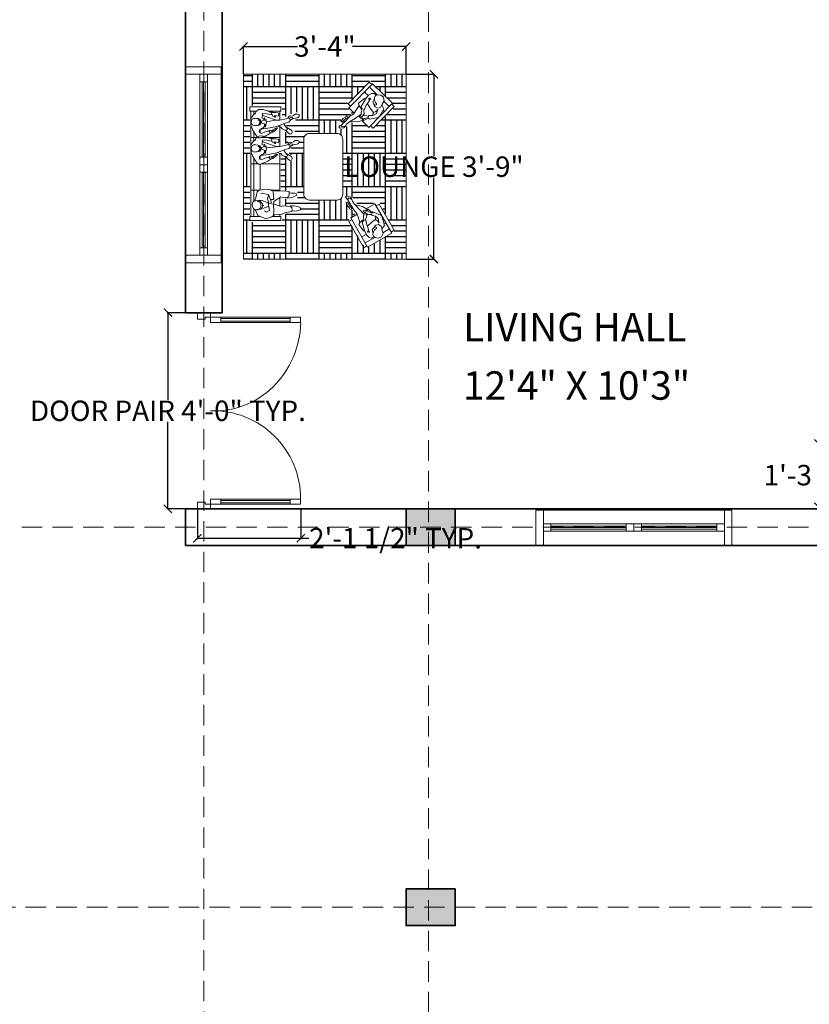
# Model space of a CAD drawing. Units: inches. Extents: x 782 to 2660, y -1008 to 166.
# Tile 3 of 12: x 1058 to 1251, y -598 to -357. Entities that reach past the tile are written whole.
import ezdxf

# ---------------------------------------------------------------- set-up
doc = ezdxf.new("R2010")
doc.units = ezdxf.units.IN
doc.header["$MEASUREMENT"] = 0
doc.linetypes.add('DASHED', pattern=[0.75, 0.5, -0.25])
for name, color, linetype, lineweight in [('A-ANNO-DIMS', 4, 'Continuous', 18), ('A-AREA-IDEN', 4, 'Continuous', 18), ('A-COLS', 7, 'Continuous', 35), ('A-Door', 150, 'Continuous', 18), ('A-FURN', 8, 'Continuous', 13), ('A-Glaz', 4, 'Continuous', 18), ('A-GRID', 8, 'DASHED', 13), ('A-WALL', 7, 'Continuous', 35)]:
    doc.layers.add(name, color=color, linetype=linetype, lineweight=lineweight)
doc.layers.add('NOITHAT', color=21, linetype='Continuous')
doc.styles.get("Standard").update_dxf_attribs({"font": 'arial.ttf'})
doc.dimstyles.get("Standard").update_dxf_attribs({"dimtxt": 5, "dimasz": 2, "dimexe": 0.18, "dimexo": 0.0625, "dimgap": 0.09, "dimtad": 0, "dimtih": 1, "dimtoh": 1, "dimdec": 0, "dimzin": 0, "dimdsep": 46, "dimlunit": 3, "dimtxsty": 'Standard', "dimblk": 'ARCHTICK', "dimcen": 0.09, "dimadec": 0, "dimazin": 0, "dimtfac": 1, "dimtdec": 0, "dimtofl": 0, "dimtmove": 0, "dimatfit": 3, "dimfxl": 1, "dimtolj": 1, "dimtzin": 0, "dimarcsym": 0})

# ---------------------------------------------------------------- blocks, each defined once
blk = doc.blocks.new('A$C13CE0A17')
at = {"layer": 'A-Door'}
for p, q in [((0, 0.61), (0, 0.69)), ((0, 0.69), (0.04, 0.69)), ((0.04, 0.69), (0.04, 0.61)), ((0, 0.61), (0, 0.08)), ((0.04, 0.61), (0, 0.61)), ((0.04, 0.61), (0, 0.61)), ((0.03, 0.61), (0.01, 0.61)), ((0.04, 0.08), (0.04, 0.61)), ((0, 0.08), (0, 0)), ((0.04, 0.08), (0, 0.08)), ((0, 0.08), (0.04, 0.08)), ((0.01, 0.08), (0.03, 0.08)), ((0.04, 0), (0.04, 0.08)), ((-0.035, 0), (-0.035, -0.1)), ((0, 0), (-0.035, 0)), ((0, 0), (0.04, 0)), ((0, -0.04), (0, 0)), ((0.015, -0.04), (0, -0.04)), ((0.015, -0.05), (0.015, -0.04)), ((0.015, -0.1), (0.015, -0.05)), ((-0.035, -0.1), (0.015, -0.1))]:
    blk.add_line(p, q, dxfattribs=at)
for points in [[(1.39, 0.69), (1.39, 0.61), (1.43, 0.61), (1.43, 0.69)], [(1.39, 0.08), (1.39, 0.61), (1.43, 0.61), (1.43, 0.08)], [(1.39, 0), (1.39, 0.08), (1.43, 0.08), (1.43, 0)], [(1.43, 0), (1.465, 0), (1.465, -0.1), (1.415, -0.1), (1.415, -0.05), (1.415, -0.04), (1.43, -0.04)]]:
    blk.add_lwpolyline(points, close=True, dxfattribs=at)
blk.add_arc((1.3872, 0.017), 0.673, 89.76573, 181.44381, dxfattribs=at)
blk.add_ellipse((0.0389, 0.0511), major_axis=(0.6669, -0.1217), ratio=0.940794, start_param=0.11153, end_param=1.73917, dxfattribs=at)
at = {"layer": 'A-Glaz'}
for p, q in [((0.01, 0.61), (0.01, 0.08)), ((0.03, 0.08), (0.03, 0.61))]:
    blk.add_line(p, q, dxfattribs=at)
blk.add_lwpolyline([(1.4, 0.08), (1.4, 0.61), (1.42, 0.61), (1.42, 0.08)], close=True, dxfattribs=at)
blk = doc.blocks.new('*X7')
at = {"color": 0}
for p, q in [((20100, 15000), (20100, 15102)), ((20200, 15000), (20200, 15102)), ((20300, 15000), (20300, 15102)), ((20400, 15000), (20400, 15102)), ((20400, 15100), (21000, 15100)), ((21000, 15000), (21000, 15102)), ((21100, 15000), (21100, 15102)), ((21200, 15000), (21200, 15102)), ((21300, 15000), (21300, 15102)), ((21400, 15000), (21400, 15102)), ((21500, 15000), (21500, 15102)), ((21600, 15000), (21600, 15102)), ((21600, 15100), (22200, 15100)), ((22200, 15000), (22200, 15102)), ((22300, 15000), (22300, 15102)), ((22400, 15000), (22400, 15102)), ((22500, 15000), (22500, 15102)), ((22600, 15000), (22600, 15102)), ((22700, 15000), (22700, 15102)), ((22800, 15000), (22800, 15102)), ((22800, 15100), (22953, 15100)), ((20023, 15000), (20400, 15000)), ((20400, 14703), (20400, 15000)), ((20400, 15000), (21000, 15000)), ((20500, 14764), (20500, 15000)), ((20600, 14825), (20600, 15000)), ((20700, 14886), (20700, 15000)), ((20800, 14850), (20800, 15000)), ((20900, 14679), (20900, 15000)), ((21000, 14509), (21000, 15000)), ((21000, 15000), (21600, 15000)), ((21600, 14400), (21600, 15000)), ((21600, 15000), (22200, 15000)), ((21700, 14400), (21700, 15000)), ((21800, 14400), (21800, 15000)), ((21900, 14400), (21900, 15000)), ((22000, 14400), (22000, 15000)), ((22100, 14400), (22100, 15000)), ((22200, 14400), (22200, 15000)), ((22200, 15000), (22800, 15000)), ((22800, 14436), (22800, 15000)), ((22800, 15000), (22953, 15000)), ((22900, 14400), (22900, 15000)), ((20023, 14900), (20400, 14900)), ((20023, 14800), (20400, 14800)), ((21000, 14900), (21600, 14900)), ((21000, 14800), (21600, 14800)), ((22200, 14900), (22800, 14900)), ((22200, 14800), (22800, 14800)), ((20023, 14700), (20395, 14700)), ((20023, 14600), (20239, 14600)), ((21000, 14700), (21600, 14700)), ((21000, 14600), (21600, 14600)), ((22200, 14700), (22800, 14700)), ((22200, 14600), (22800, 14600)), ((20023, 14500), (20290, 14500)), ((20023, 14400), (20341, 14400)), ((20100, 13800), (20100, 14400)), ((20200, 13800), (20200, 14400)), ((20300, 13800), (20300, 14400)), ((21005, 14500), (21600, 14500)), ((21048, 14400), (21600, 14400)), ((21100, 14103), (21100, 14400)), ((21200, 14013), (21200, 14400)), ((21300, 14038), (21300, 14400)), ((21400, 14038), (21400, 14400)), ((21500, 14038), (21500, 14400)), ((21600, 14038), (21600, 14400)), ((21600, 14400), (22200, 14400)), ((22200, 14500), (22800, 14500)), ((22200, 14301), (22200, 14400)), ((22200, 14400), (22258, 14400)), ((22840, 14400), (22953, 14400)), ((20400, 13800), (20400, 14284)), ((20400, 14200), (20443, 14200)), ((20948, 14300), (21000, 14300)), ((21000, 14220), (21000, 14352)), ((21600, 14300), (22196, 14300)), ((21600, 14200), (21914, 14200)), ((22840, 14300), (22953, 14300)), ((22840, 14200), (22953, 14200)), ((20400, 14100), (20493, 14100)), ((20615, 14100), (20911, 14100)), ((21600, 14100), (22200, 14100)), ((22200, 14013), (22200, 14136)), ((22840, 14100), (22953, 14100)), ((20400, 14000), (20986, 14000)), ((20400, 13900), (21000, 13900)), ((21000, 13800), (21000, 13985)), ((21100, 13800), (21100, 13955)), ((21846, 14000), (21984, 14000)), ((21867, 13900), (21984, 13900)), ((22200, 13800), (22200, 13872)), ((22840, 14000), (22953, 14000)), ((22840, 13900), (22953, 13900)), ((20023, 13800), (20400, 13800)), ((20023, 13700), (20400, 13700)), ((20400, 13200), (20400, 13800)), ((20400, 13800), (21000, 13800)), ((20500, 13200), (20500, 13800)), ((20600, 13200), (20600, 13800)), ((20700, 13200), (20700, 13800)), ((20800, 13200), (20800, 13800)), ((20900, 13200), (20900, 13800)), ((21000, 13200), (21000, 13800)), ((21000, 13800), (21167, 13800)), ((21000, 13700), (21167, 13700)), ((21867, 13800), (22200, 13800)), ((21900, 13200), (21900, 13800)), ((22000, 13200), (22000, 13800)), ((22100, 13337), (22100, 13800)), ((22200, 13278), (22200, 13800)), ((22200, 13800), (22284, 13800)), ((22200, 13700), (22284, 13700)), ((22840, 13800), (22953, 13800)), ((22900, 13200), (22900, 13800)), ((20023, 13600), (20400, 13600)), ((20023, 13500), (20400, 13500)), ((21000, 13600), (21167, 13600)), ((21000, 13500), (21167, 13500)), ((22200, 13600), (22284, 13600)), ((22200, 13500), (22284, 13500)), ((20023, 13400), (20400, 13400)), ((21000, 13400), (21167, 13400)), ((22200, 13400), (22284, 13400)), ((20023, 13300), (20400, 13300)), ((20023, 13200), (20400, 13200)), ((20100, 12600), (20100, 13200)), ((20200, 12600), (20200, 13200)), ((20300, 12600), (20300, 13200)), ((20400, 12600), (20400, 13200)), ((20400, 13200), (21000, 13200)), ((21000, 13300), (21167, 13300)), ((21000, 12645), (21000, 13200)), ((21000, 13200), (21167, 13200)), ((21100, 12710), (21100, 13200)), ((21867, 13200), (22129, 13200)), ((22100, 13200), (22100, 13222)), ((22200, 13300), (22284, 13300)), ((22840, 13200), (22953, 13200)), ((20400, 13100), (21000, 13100)), ((20400, 13000), (21000, 13000)), ((21867, 13100), (22104, 13100)), ((21867, 13000), (21940, 13000)), ((22158, 13000), (22200, 13000)), ((22200, 12812), (22200, 13017)), ((22840, 13100), (22953, 13100)), ((22840, 13000), (22953, 13000)), ((20400, 12900), (21000, 12900)), ((20400, 12800), (21000, 12800)), ((21200, 12760), (21200, 12864)), ((21300, 12600), (21300, 12838)), ((21400, 12600), (21400, 12838)), ((21500, 12600), (21500, 12838)), ((21600, 12600), (21600, 12838)), ((21600, 12800), (22032, 12800)), ((21859, 12900), (22200, 12900)), ((22840, 12900), (22953, 12900)), ((22840, 12800), (22953, 12800)), ((20023, 12600), (20400, 12600)), ((20400, 12700), (20570, 12700)), ((20400, 12536), (20400, 12600)), ((20400, 12600), (20466, 12600)), ((20745, 12700), (21000, 12700)), ((21194, 12600), (21600, 12600)), ((21200, 12600), (21200, 12607)), ((21600, 12700), (22177, 12700)), ((21600, 12000), (21600, 12600)), ((21600, 12600), (22019, 12600)), ((21700, 12000), (21700, 12600)), ((21800, 12000), (21800, 12600)), ((21900, 12000), (21900, 12600)), ((22000, 12592), (22000, 12600)), ((22840, 12700), (22953, 12700)), ((22840, 12600), (22953, 12600)), ((22900, 12000), (22900, 12600)), ((20023, 12500), (20362, 12500)), ((21000, 12457), (21000, 12480)), ((21025, 12500), (21600, 12500)), ((22000, 12000), (22000, 12457)), ((22100, 12000), (22100, 12483)), ((22200, 12000), (22200, 12534)), ((22200, 12500), (22258, 12500)), ((20023, 12400), (20258, 12400)), ((20023, 12300), (20265, 12300)), ((21057, 12400), (21600, 12400)), ((21082, 12300), (21600, 12300)), ((22200, 12400), (22258, 12400)), ((22200, 12300), (22800, 12300)), ((22800, 12000), (22800, 12337)), ((20023, 12200), (20363, 12200)), ((20023, 12100), (20400, 12100)), ((20400, 12000), (20400, 12163)), ((20900, 12000), (20900, 12118)), ((21000, 12000), (21000, 12218)), ((21000, 12200), (21600, 12200)), ((21000, 12100), (21600, 12100)), ((22200, 12200), (22800, 12200)), ((22200, 12100), (22800, 12100)), ((20023, 12000), (20400, 12000)), ((20100, 11772), (20100, 12000)), ((20200, 11772), (20200, 12000)), ((20300, 11772), (20300, 12000)), ((20400, 11772), (20400, 12000)), ((20400, 12000), (20560, 12000)), ((20400, 11900), (20658, 11900)), ((20500, 12000), (20500, 12061)), ((20682, 11900), (21000, 11900)), ((20782, 12000), (21000, 12000)), ((20800, 12000), (20800, 12018)), ((21000, 11772), (21000, 12000)), ((21000, 12000), (21600, 12000)), ((21100, 11772), (21100, 12000)), ((21200, 11772), (21200, 12000)), ((21300, 11772), (21300, 12000)), ((21400, 11772), (21400, 12000)), ((21500, 11772), (21500, 12000)), ((21600, 11772), (21600, 12000)), ((21600, 12000), (22200, 12000)), ((21600, 11900), (22200, 11900)), ((22200, 11772), (22200, 12000)), ((22200, 12000), (22800, 12000)), ((22300, 11772), (22300, 12000)), ((22400, 11772), (22400, 12000)), ((22500, 11772), (22500, 12000)), ((22600, 11772), (22600, 12000)), ((22700, 11772), (22700, 12000)), ((22800, 11772), (22800, 12000)), ((22800, 12000), (22953, 12000)), ((22800, 11900), (22953, 11900)), ((20400, 11800), (21000, 11800)), ((21600, 11800), (22200, 11800)), ((22800, 11800), (22953, 11800))]:
    blk.add_line(p, q, dxfattribs=at)
blk = doc.blocks.new('A$C47115F23')
at = {"linetype": 'ByBlock'}
for p, q in [((693, 2256), (693, 2818)), ((693, 2818), (768, 2818)), ((728, 2530), (788, 2676)), ((768, 2629), (768, 2818)), ((768, 2800), (2668, 2800)), ((768, 2743), (908, 2743)), ((788, 2676), (884, 2718)), ((890, 2723), (888, 2688)), ((888, 2688), (898, 2620)), ((890, 2723), (914, 2751)), ((892, 2687), (904, 2639)), ((914, 2751), (946, 2771)), ((946, 2771), (985, 2775)), ((985, 2775), (1037, 2759)), ((1027, 2639), (1039, 2683)), ((1039, 2683), (1035, 2648)), ((1056, 2700), (1037, 2759)), ((1042, 2743), (1815, 2743)), ((1049, 2650), (1056, 2700)), ((1072, 2723), (1050, 2729)), ((1056, 2593), (1061, 2665)), ((1072, 2723), (1104, 2707)), ((1104, 2707), (1210, 2684)), ((1210, 2684), (1242, 2652)), ((1243, 2800), (1243, 2644)), ((1710, 2662), (1709, 2626)), ((1729, 2684), (1710, 2662)), ((1718, 2800), (1718, 2671)), ((1790, 2728), (1729, 2684)), ((1846, 2763), (1790, 2728)), ((1893, 2783), (1846, 2763)), ((1939, 2797), (1893, 2783)), ((1928, 2739), (1930, 2714)), ((1932, 2739), (1928, 2739)), ((1930, 2714), (1932, 2685)), ((1933, 2750), (1932, 2739)), ((1932, 2685), (1939, 2656)), ((1942, 2777), (1933, 2750)), ((1979, 2802), (1939, 2797)), ((1952, 2655), (1940, 2668)), ((1964, 2790), (1942, 2777)), ((1994, 2795), (1964, 2790)), ((2047, 2799), (1979, 2802)), ((2021, 2790), (1994, 2795)), ((2045, 2777), (2021, 2790)), ((2030, 2672), (2026, 2650)), ((2036, 2650), (2030, 2672)), ((2042, 2640), (2056, 2669)), ((2055, 2756), (2045, 2777)), ((2082, 2783), (2047, 2799)), ((2059, 2741), (2055, 2756)), ((2056, 2669), (2059, 2712)), ((2064, 2736), (2059, 2741)), ((2059, 2712), (2064, 2736)), ((2118, 2755), (2082, 2783)), ((2152, 2716), (2118, 2755)), ((2127, 2743), (2290, 2743)), ((2179, 2707), (2152, 2716)), ((2196, 2692), (2179, 2707)), ((2185, 2662), (2184, 2626)), ((2204, 2684), (2185, 2662)), ((2193, 2800), (2193, 2694)), ((2193, 2800), (2193, 2671)), ((2218, 2658), (2196, 2692)), ((2265, 2728), (2204, 2684)), ((2321, 2763), (2265, 2728)), ((2368, 2783), (2321, 2763)), ((2414, 2797), (2368, 2783)), ((2403, 2739), (2405, 2714)), ((2407, 2739), (2403, 2739)), ((2405, 2714), (2407, 2685)), ((2408, 2750), (2407, 2739)), ((2407, 2685), (2414, 2656)), ((2417, 2777), (2408, 2750)), ((2454, 2802), (2414, 2797)), ((2427, 2655), (2415, 2668)), ((2439, 2790), (2417, 2777)), ((2469, 2795), (2439, 2790)), ((2522, 2799), (2454, 2802)), ((2496, 2790), (2469, 2795)), ((2520, 2777), (2496, 2790)), ((2505, 2672), (2501, 2650)), ((2511, 2650), (2505, 2672)), ((2517, 2640), (2531, 2669)), ((2530, 2756), (2520, 2777)), ((2557, 2783), (2522, 2799)), ((2534, 2741), (2530, 2756)), ((2531, 2669), (2534, 2712)), ((2539, 2736), (2534, 2741)), ((2534, 2712), (2539, 2736)), ((2593, 2755), (2557, 2783)), ((2627, 2716), (2593, 2755)), ((2602, 2743), (2668, 2743)), ((2654, 2707), (2627, 2716)), ((2671, 2692), (2654, 2707)), ((2668, 2818), (2668, 2694)), ((2668, 2818), (2743, 2818)), ((2693, 2658), (2671, 2692)), ((2743, 2818), (2743, 2256)), ((760, 2423), (728, 2530)), ((768, 2631), (769, 2631)), ((867, 2553), (843, 2518)), ((843, 2518), (874, 2463)), ((874, 2463), (1011, 2485)), ((896, 2631), (921, 2631)), ((898, 2620), (927, 2598)), ((904, 2639), (960, 2612)), ((911, 2583), (946, 2485)), ((927, 2598), (955, 2589)), ((955, 2589), (963, 2573)), ((960, 2612), (1003, 2624)), ((963, 2573), (968, 2573)), ((968, 2573), (977, 2590)), ((977, 2590), (1002, 2598)), ((1011, 2485), (989, 2391)), ((1002, 2598), (1031, 2619)), ((1003, 2624), (1027, 2639)), ((1011, 2476), (1056, 2593)), ((1088, 2498), (1011, 2476)), ((1014, 2631), (1059, 2631)), ((1031, 2619), (1049, 2650)), ((1035, 2648), (1043, 2643)), ((1155, 2482), (1088, 2498)), ((1163, 2482), (1187, 2621)), ((1242, 2652), (1262, 2530)), ((1246, 2631), (1718, 2631)), ((1262, 2530), (1250, 2447)), ((1709, 2626), (1742, 2555)), ((1718, 2605), (1718, 2275)), ((1742, 2555), (1764, 2496)), ((1764, 2496), (1783, 2467)), ((1786, 2616), (1802, 2640)), ((1803, 2584), (1786, 2616)), ((1796, 2631), (1860, 2631)), ((1802, 2640), (1825, 2648)), ((1827, 2524), (1803, 2584)), ((1825, 2648), (1849, 2646)), ((1832, 2494), (1827, 2524)), ((1829, 2482), (1832, 2494)), ((1849, 2646), (1874, 2612)), ((1883, 2606), (1869, 2602)), ((1869, 2602), (1871, 2575)), ((1871, 2575), (1879, 2526)), ((1874, 2612), (1883, 2606)), ((1879, 2592), (1881, 2599)), ((1896, 2574), (1879, 2592)), ((1879, 2526), (1915, 2333)), ((1923, 2553), (1896, 2574)), ((1933, 2530), (1903, 2545)), ((1957, 2553), (1923, 2553)), ((1952, 2536), (1933, 2530)), ((1939, 2656), (1947, 2638)), ((1947, 2638), (1962, 2626)), ((1972, 2642), (1952, 2655)), ((1956, 2631), (2028, 2631)), ((1957, 2540), (1979, 2614)), ((1959, 2523), (1957, 2540)), ((1972, 2629), (1959, 2635)), ((2003, 2516), (1959, 2523)), ((1962, 2626), (1981, 2622)), ((1996, 2638), (1972, 2642)), ((1981, 2622), (1990, 2608)), ((1990, 2608), (1998, 2609)), ((2013, 2641), (1996, 2638)), ((1998, 2609), (2005, 2624)), ((2035, 2538), (2003, 2516)), ((2005, 2624), (2023, 2628)), ((2010, 2455), (2005, 2513)), ((2029, 2635), (2008, 2630)), ((2026, 2650), (2013, 2641)), ((2013, 2623), (2016, 2590)), ((2016, 2590), (2025, 2560)), ((2018, 2528), (2040, 2521)), ((2023, 2628), (2042, 2640)), ((2025, 2560), (2033, 2555)), ((2057, 2580), (2033, 2567)), ((2033, 2555), (2035, 2538)), ((2050, 2660), (2036, 2650)), ((2040, 2541), (2055, 2546)), ((2043, 2379), (2113, 2584)), ((2055, 2546), (2069, 2558)), ((2072, 2599), (2057, 2580)), ((2087, 2596), (2072, 2599)), ((2111, 2589), (2087, 2596)), ((2113, 2584), (2128, 2594)), ((2141, 2519), (2125, 2428)), ((2128, 2594), (2148, 2585)), ((2148, 2585), (2141, 2519)), ((2184, 2626), (2217, 2555)), ((2190, 2482), (2218, 2577)), ((2193, 2605), (2193, 2275)), ((2193, 2492), (2193, 2275)), ((2217, 2555), (2239, 2496)), ((2223, 2616), (2218, 2658)), ((2218, 2577), (2223, 2616)), ((2239, 2496), (2258, 2467)), ((2261, 2616), (2277, 2640)), ((2278, 2584), (2261, 2616)), ((2271, 2631), (2335, 2631)), ((2277, 2640), (2300, 2648)), ((2302, 2524), (2278, 2584)), ((2300, 2648), (2324, 2646)), ((2307, 2494), (2302, 2524)), ((2304, 2482), (2307, 2494)), ((2324, 2646), (2349, 2612)), ((2358, 2606), (2344, 2602)), ((2344, 2602), (2346, 2575)), ((2346, 2575), (2354, 2526)), ((2349, 2612), (2358, 2606)), ((2354, 2592), (2356, 2599)), ((2371, 2574), (2354, 2592)), ((2354, 2526), (2390, 2333)), ((2398, 2553), (2371, 2574)), ((2408, 2530), (2378, 2545)), ((2432, 2553), (2398, 2553)), ((2427, 2536), (2408, 2530)), ((2414, 2656), (2422, 2638)), ((2422, 2638), (2437, 2626)), ((2447, 2642), (2427, 2655)), ((2431, 2631), (2503, 2631)), ((2432, 2540), (2454, 2614)), ((2434, 2523), (2432, 2540)), ((2447, 2629), (2434, 2635)), ((2478, 2516), (2434, 2523)), ((2437, 2626), (2456, 2622)), ((2471, 2638), (2447, 2642)), ((2456, 2622), (2465, 2608)), ((2465, 2608), (2473, 2609)), ((2488, 2641), (2471, 2638)), ((2473, 2609), (2480, 2624)), ((2510, 2538), (2478, 2516)), ((2480, 2624), (2498, 2628)), ((2485, 2455), (2480, 2513)), ((2504, 2635), (2483, 2630)), ((2501, 2650), (2488, 2641)), ((2488, 2623), (2491, 2590)), ((2491, 2590), (2500, 2560)), ((2493, 2528), (2515, 2521)), ((2498, 2628), (2517, 2640)), ((2500, 2560), (2508, 2555)), ((2532, 2580), (2508, 2567)), ((2508, 2555), (2510, 2538)), ((2525, 2660), (2511, 2650)), ((2515, 2541), (2530, 2546)), ((2518, 2379), (2588, 2584)), ((2530, 2546), (2544, 2558)), ((2547, 2599), (2532, 2580)), ((2562, 2596), (2547, 2599)), ((2586, 2589), (2562, 2596)), ((2588, 2584), (2603, 2594)), ((2616, 2519), (2600, 2428)), ((2603, 2594), (2623, 2585)), ((2623, 2585), (2616, 2519)), ((2665, 2482), (2693, 2577)), ((2668, 2492), (2668, 2256)), ((2698, 2616), (2693, 2658)), ((2693, 2577), (2698, 2616)), ((795, 2376), (760, 2423)), ((768, 2256), (768, 2412)), ((851, 2384), (795, 2391)), ((811, 2241), (795, 2376)), ((989, 2391), (851, 2384)), ((993, 2388), (950, 2245)), ((1040, 2388), (993, 2388)), ((1068, 2439), (1013, 2435)), ((1120, 2257), (1040, 2388)), ((1072, 2388), (1076, 2443)), ((1210, 2399), (1072, 2388)), ((1076, 2443), (1163, 2482)), ((1230, 2415), (1222, 2301)), ((1250, 2447), (1230, 2415)), ((1243, 2436), (1243, 2275)), ((1783, 2467), (1797, 2442)), ((1797, 2442), (1805, 2440)), ((1803, 2443), (1808, 2457)), ((1805, 2440), (1813, 2403)), ((1808, 2457), (1822, 2464)), ((1813, 2403), (1846, 2355)), ((1830, 2419), (1819, 2423)), ((1822, 2464), (1837, 2458)), ((1839, 2469), (1829, 2482)), ((1838, 2407), (1830, 2419)), ((1835, 2447), (1846, 2453)), ((1842, 2435), (1835, 2447)), ((1844, 2401), (1838, 2407)), ((1846, 2453), (1839, 2469)), ((1849, 2418), (1842, 2435)), ((1849, 2405), (1844, 2401)), ((1846, 2355), (1886, 2320)), ((1851, 2408), (1849, 2418)), ((1857, 2389), (1851, 2408)), ((1876, 2355), (1857, 2389)), ((1888, 2338), (1876, 2355)), ((1891, 2325), (1879, 2340)), ((1879, 2340), (1888, 2338)), ((1886, 2320), (1891, 2325)), ((1901, 2277), (1915, 2308)), ((1915, 2333), (1942, 2262)), ((2020, 2384), (2010, 2455)), ((2028, 2326), (2020, 2384)), ((2030, 2330), (2043, 2379)), ((2030, 2277), (2030, 2330)), ((2103, 2404), (2084, 2365)), ((2084, 2365), (2084, 2355)), ((2084, 2355), (2089, 2354)), ((2089, 2354), (2108, 2372)), ((2128, 2413), (2103, 2404)), ((2114, 2372), (2103, 2301)), ((2108, 2372), (2114, 2372)), ((2125, 2428), (2128, 2413)), ((2131, 2426), (2147, 2429)), ((2147, 2429), (2171, 2413)), ((2162, 2306), (2165, 2350)), ((2165, 2350), (2167, 2404)), ((2167, 2404), (2175, 2408)), ((2175, 2452), (2190, 2482)), ((2175, 2408), (2175, 2452)), ((2258, 2467), (2272, 2442)), ((2272, 2442), (2280, 2440)), ((2278, 2443), (2283, 2457)), ((2280, 2440), (2288, 2403)), ((2283, 2457), (2297, 2464)), ((2288, 2403), (2321, 2355)), ((2305, 2419), (2294, 2423)), ((2297, 2464), (2312, 2458)), ((2314, 2469), (2304, 2482)), ((2313, 2407), (2305, 2419)), ((2310, 2447), (2321, 2453)), ((2317, 2435), (2310, 2447)), ((2319, 2401), (2313, 2407)), ((2321, 2453), (2314, 2469)), ((2324, 2418), (2317, 2435)), ((2324, 2405), (2319, 2401)), ((2321, 2355), (2361, 2320)), ((2326, 2408), (2324, 2418)), ((2332, 2389), (2326, 2408)), ((2351, 2355), (2332, 2389)), ((2363, 2338), (2351, 2355)), ((2366, 2325), (2354, 2340)), ((2354, 2340), (2363, 2338)), ((2361, 2320), (2366, 2325)), ((2376, 2277), (2390, 2308)), ((2390, 2333), (2417, 2262)), ((2495, 2384), (2485, 2455)), ((2503, 2326), (2495, 2384)), ((2505, 2330), (2518, 2379)), ((2505, 2277), (2505, 2330)), ((2578, 2404), (2559, 2365)), ((2559, 2365), (2559, 2355)), ((2559, 2355), (2564, 2354)), ((2564, 2354), (2583, 2372)), ((2603, 2413), (2578, 2404)), ((2589, 2372), (2578, 2301)), ((2583, 2372), (2589, 2372)), ((2600, 2428), (2603, 2413)), ((2606, 2426), (2622, 2429)), ((2622, 2429), (2646, 2413)), ((2637, 2306), (2640, 2350)), ((2640, 2350), (2642, 2404)), ((2642, 2404), (2650, 2408)), ((2650, 2452), (2665, 2482)), ((2650, 2408), (2650, 2452)), ((768, 2256), (693, 2256)), ((807, 2275), (768, 2275)), ((835, 2186), (811, 2241)), ((859, 2068), (835, 2186)), ((950, 2245), (957, 2222)), ((957, 2222), (950, 2091)), ((1109, 2275), (959, 2275)), ((1096, 2135), (1116, 2151)), ((1116, 2044), (1096, 2135)), ((1112, 2230), (1120, 2257)), ((1116, 2151), (1112, 2230)), ((1124, 2123), (1112, 2170)), ((1230, 2210), (1218, 2111)), ((1222, 2301), (1230, 2210)), ((1902, 2275), (1225, 2275)), ((1798, 2125), (1830, 2156)), ((1830, 2156), (1844, 2172)), ((1896, 2150), (1844, 2062)), ((1846, 2186), (1871, 2232)), ((1846, 2157), (1846, 2186)), ((1856, 2147), (1846, 2157)), ((1874, 2140), (1856, 2147)), ((1871, 2232), (1903, 2260)), ((1901, 2161), (1874, 2140)), ((1903, 2260), (1901, 2277)), ((1959, 2206), (1901, 2161)), ((1942, 2262), (1967, 2198)), ((1967, 2198), (1993, 2112)), ((2054, 2164), (2030, 2277)), ((2412, 2275), (2030, 2275)), ((2065, 2125), (2054, 2164)), ((2103, 2301), (2113, 2301)), ((2113, 2301), (2118, 2284)), ((2118, 2284), (2123, 2288)), ((2123, 2288), (2131, 2296)), ((2131, 2296), (2141, 2298)), ((2141, 2298), (2147, 2303)), ((2147, 2303), (2162, 2306)), ((2273, 2125), (2305, 2156)), ((2305, 2156), (2319, 2172)), ((2371, 2150), (2319, 2062)), ((2321, 2186), (2346, 2232)), ((2321, 2157), (2321, 2186)), ((2331, 2147), (2321, 2157)), ((2349, 2140), (2331, 2147)), ((2346, 2232), (2378, 2260)), ((2376, 2161), (2349, 2140)), ((2378, 2260), (2376, 2277)), ((2434, 2206), (2376, 2161)), ((2417, 2262), (2442, 2198)), ((2442, 2198), (2468, 2112)), ((2529, 2164), (2505, 2277)), ((2668, 2275), (2505, 2275)), ((2540, 2125), (2529, 2164)), ((2578, 2301), (2588, 2301)), ((2588, 2301), (2593, 2284)), ((2593, 2284), (2598, 2288)), ((2598, 2288), (2606, 2296)), ((2606, 2296), (2616, 2298)), ((2616, 2298), (2622, 2303)), ((2622, 2303), (2637, 2306)), ((2668, 2256), (2743, 2256)), ((874, 2056), (859, 2068)), ((889, 1903), (861, 1982)), ((863, 1981), (867, 2044)), ((867, 2044), (874, 2056)), ((924, 2063), (894, 2054)), ((946, 1953), (922, 1902)), ((945, 2083), (924, 2063)), ((957, 2032), (946, 1953)), ((950, 2091), (957, 2079)), ((957, 2079), (957, 2032)), ((1151, 1969), (1116, 2044)), ((1159, 2107), (1124, 2123)), ((1179, 1977), (1151, 1969)), ((1191, 2107), (1159, 2107)), ((1187, 2008), (1179, 1977)), ((1195, 2107), (1187, 2068)), ((1187, 2068), (1187, 2008)), ((1218, 2111), (1195, 2107)), ((1778, 2096), (1798, 2125)), ((1783, 2069), (1778, 2096)), ((1808, 2052), (1783, 2069)), ((1844, 2062), (1808, 2052)), ((1993, 2112), (2030, 2086)), ((2030, 2086), (2055, 2049)), ((2042, 2090), (2057, 2105)), ((2055, 2049), (2059, 2025)), ((2057, 2105), (2062, 2120)), ((2057, 2040), (2074, 2056)), ((2059, 2025), (2076, 1946)), ((2082, 2125), (2065, 2125)), ((2079, 2091), (2070, 2103)), ((2074, 2056), (2081, 2076)), ((2081, 2076), (2079, 2091)), ((2099, 2106), (2082, 2125)), ((2109, 2076), (2099, 2106)), ((2103, 2069), (2109, 2076)), ((2113, 2032), (2103, 2069)), ((2135, 2000), (2113, 2032)), ((2128, 1929), (2138, 1954)), ((2138, 1954), (2135, 2000)), ((2253, 2096), (2273, 2125)), ((2258, 2069), (2253, 2096)), ((2283, 2052), (2258, 2069)), ((2319, 2062), (2283, 2052)), ((2468, 2112), (2505, 2086)), ((2505, 2086), (2530, 2049)), ((2517, 2090), (2532, 2105)), ((2530, 2049), (2534, 2025)), ((2532, 2105), (2537, 2120)), ((2532, 2040), (2549, 2056)), ((2534, 2025), (2551, 1946)), ((2557, 2125), (2540, 2125)), ((2554, 2091), (2545, 2103)), ((2549, 2056), (2556, 2076)), ((2556, 2076), (2554, 2091)), ((2574, 2106), (2557, 2125)), ((2584, 2076), (2574, 2106)), ((2578, 2069), (2584, 2076)), ((2588, 2032), (2578, 2069)), ((2610, 2000), (2588, 2032)), ((2603, 1929), (2613, 1954)), ((2613, 1954), (2610, 2000)), ((922, 1902), (890, 1902)), ((2076, 1946), (2101, 1927)), ((2101, 1927), (2128, 1929)), ((2551, 1946), (2576, 1927)), ((2576, 1927), (2603, 1929)), ((1023, 1080), (953, 1052)), ((1025, 1059), (1023, 1080)), ((1093, 1075), (1069, 1049)), ((1120, 1091), (1093, 1075)), ((1114, 1001), (1142, 1069)), ((1142, 1069), (1120, 1091)), ((2357, 1196), (2383, 1212)), ((2367, 1123), (2357, 1196)), ((2387, 1102), (2367, 1123)), ((2383, 1212), (2406, 1190)), ((2395, 1164), (2386, 1156)), ((2386, 1156), (2390, 1128)), ((2406, 1090), (2387, 1102)), ((2390, 1128), (2402, 1088)), ((2414, 1159), (2395, 1164)), ((2406, 1190), (2422, 1158)), ((2429, 1075), (2406, 1090)), ((2422, 1158), (2448, 1136)), ((2471, 1023), (2429, 1075)), ((2448, 1136), (2479, 1101)), ((2468, 1157), (2475, 1177)), ((2483, 1131), (2468, 1157)), ((2475, 1177), (2536, 1133)), ((2479, 1101), (2483, 1131)), ((2547, 1039), (2479, 1101)), ((2533, 1090), (2491, 1130)), ((2549, 1052), (2533, 1090)), ((2536, 1133), (2560, 1094)), ((2560, 1094), (2581, 1077)), ((2581, 1077), (2570, 1052)), ((678, 1034), (205, 761)), ((746, 1000), (218, 696)), ((710, 979), (678, 1034)), ((812, 885), (746, 1000)), ((824, 889), (759, 867)), ((886, 946), (824, 889)), ((919, 964), (886, 946)), ((892, 841), (988, 930)), ((919, 1020), (895, 1009)), ((895, 1009), (900, 983)), ((900, 983), (919, 964)), ((953, 1052), (919, 1020)), ((919, 964), (999, 1007)), ((920, 977), (945, 1010)), ((945, 1010), (995, 1039)), ((960, 842), (980, 912)), ((980, 912), (988, 930)), ((988, 930), (1042, 969)), ((999, 1007), (1003, 1037)), ((1039, 1034), (999, 1007)), ((1003, 1037), (1025, 1059)), ((1069, 1049), (1039, 1034)), ((1042, 969), (1068, 978)), ((1068, 978), (1089, 985)), ((1093, 1011), (1071, 976)), ((1078, 1047), (1097, 1047)), ((1089, 985), (1114, 1001)), ((1103, 1037), (1093, 1011)), ((1097, 1047), (1103, 1037)), ((2475, 1004), (2471, 1023)), ((2542, 914), (2472, 1023)), ((2477, 931), (2475, 1004)), ((2475, 877), (2477, 931)), ((2604, 816), (2542, 914)), ((2570, 1052), (2547, 1039)), ((2547, 1039), (2574, 1013)), ((2574, 1013), (2620, 942)), ((2620, 942), (2677, 905)), ((2630, 936), (2723, 1031)), ((2677, 905), (2770, 850)), ((2723, 1031), (3159, 606)), ((2753, 1002), (2797, 1047)), ((2797, 1047), (3188, 665)), ((205, 761), (237, 707)), ((291, 738), (389, 568)), ((436, 718), (392, 666)), ((446, 722), (400, 801)), ((503, 748), (436, 718)), ((510, 771), (503, 748)), ((623, 856), (510, 771)), ((664, 792), (518, 750)), ((534, 677), (621, 710)), ((621, 710), (708, 725)), ((655, 836), (623, 856)), ((759, 867), (655, 836)), ((664, 830), (709, 776)), ((697, 766), (664, 792)), ((770, 768), (697, 766)), ((704, 738), (809, 700)), ((708, 725), (704, 738)), ((848, 752), (770, 768)), ((790, 720), (850, 736)), ((819, 707), (790, 720)), ((808, 763), (892, 841)), ((838, 783), (855, 774)), ((850, 736), (848, 752)), ((855, 774), (874, 755)), ((869, 730), (861, 713)), ((861, 713), (887, 722)), ((893, 717), (862, 689)), ((874, 755), (869, 730)), ((887, 722), (893, 717)), ((893, 698), (948, 789)), ((998, 564), (907, 721)), ((948, 789), (960, 842)), ((2371, 671), (2498, 801)), ((2506, 775), (2475, 877)), ((2497, 767), (2506, 775)), ((2540, 675), (2497, 767)), ((2518, 796), (2511, 793)), ((2511, 793), (2534, 758)), ((2540, 781), (2518, 796)), ((2534, 758), (2549, 683)), ((2538, 826), (2537, 800)), ((2537, 800), (2540, 781)), ((2561, 839), (2538, 826)), ((2557, 801), (2563, 816)), ((2611, 770), (2557, 801)), ((2580, 843), (2561, 839)), ((2563, 816), (2642, 812)), ((2576, 677), (2585, 735)), ((2580, 765), (2611, 770)), ((2588, 756), (2580, 765)), ((2699, 766), (2588, 756)), ((2642, 812), (2712, 793)), ((2691, 755), (2699, 766)), ((2772, 719), (2691, 755)), ((2760, 846), (2703, 805)), ((2712, 793), (2751, 809)), ((2751, 809), (2882, 733)), ((2770, 850), (2807, 861)), ((2848, 665), (2772, 719)), ((2807, 861), (2895, 751)), ((2895, 751), (2896, 727)), ((2896, 727), (2953, 681)), ((2945, 687), (3009, 752)), ((218, 696), (470, 260)), ((389, 568), (377, 502)), ((392, 666), (379, 624)), ((379, 624), (399, 575)), ((399, 575), (389, 568)), ((423, 595), (404, 581)), ((452, 601), (423, 595)), ((486, 590), (452, 601)), ((469, 598), (532, 612)), ((470, 260), (998, 564)), ((475, 669), (511, 666)), ((511, 666), (485, 700)), ((485, 700), (534, 677)), ((529, 571), (486, 590)), ((550, 536), (529, 571)), ((532, 612), (566, 581)), ((567, 533), (550, 536)), ((566, 581), (579, 562)), ((586, 571), (567, 533)), ((611, 547), (586, 571)), ((591, 695), (672, 615)), ((623, 500), (611, 547)), ((672, 615), (715, 553)), ((715, 553), (688, 517)), ((715, 553), (769, 555)), ((720, 497), (772, 552)), ((772, 552), (792, 623)), ((779, 437), (850, 598)), ((792, 623), (818, 613)), ((801, 621), (806, 679)), ((809, 700), (819, 707)), ((862, 689), (828, 619)), ((835, 609), (899, 688)), ((850, 598), (835, 609)), ((899, 688), (893, 698)), ((993, 488), (961, 543)), ((2357, 596), (2401, 641)), ((2748, 215), (2357, 596)), ((2807, 245), (2371, 671)), ((2523, 667), (2540, 675)), ((2551, 494), (2523, 667)), ((2585, 677), (2557, 674)), ((2587, 604), (2585, 677)), ((2623, 537), (2587, 604)), ((2642, 590), (2590, 605)), ((2695, 514), (2623, 537)), ((2699, 639), (2642, 590)), ((2642, 590), (2660, 548)), ((2660, 548), (2695, 514)), ((2798, 697), (2699, 639)), ((2719, 516), (2742, 558)), ((2742, 558), (2771, 575)), ((2771, 575), (2781, 534)), ((2794, 581), (2776, 565)), ((2781, 534), (2798, 533)), ((2834, 602), (2794, 581)), ((2798, 533), (2827, 562)), ((3159, 606), (2807, 245)), ((2827, 562), (2873, 569)), ((2892, 573), (2834, 602)), ((2902, 676), (2848, 665)), ((2868, 649), (2902, 676)), ((2903, 643), (2868, 649)), ((2873, 569), (2909, 572)), ((2909, 572), (2935, 558)), ((2935, 558), (2951, 540)), ((2953, 681), (2983, 620)), ((2985, 575), (2954, 533)), ((2954, 533), (2962, 524)), ((3099, 664), (2962, 524)), ((2983, 620), (2985, 575)), ((3188, 665), (3144, 620)), ((377, 502), (400, 446)), ((400, 446), (464, 416)), ((464, 416), (534, 439)), ((474, 420), (543, 301)), ((520, 215), (993, 488)), ((534, 439), (553, 434)), ((540, 435), (596, 453)), ((553, 434), (605, 390)), ((596, 453), (623, 500)), ((605, 390), (779, 437)), ((652, 364), (633, 397)), ((688, 517), (645, 492)), ((645, 492), (720, 497)), ((2708, 405), (2551, 494)), ((2656, 392), (2683, 419)), ((2769, 435), (2708, 405)), ((2732, 464), (2719, 516)), ((2783, 432), (2732, 464)), ((2842, 402), (2747, 304)), ((2790, 435), (2769, 435)), ((2852, 396), (2790, 435)), ((2920, 408), (2852, 396)), ((2957, 457), (2920, 408)), ((2962, 524), (2957, 457)), ((488, 270), (520, 215)), ((2792, 260), (2748, 215))]:
    blk.add_line(p, q, dxfattribs=at)
blk.add_lwpolyline([(0, 0), (3331, 0), (3331, 2930), (0, 2930)], close=True)
blk.add_lwpolyline([(2264, 1244), (2264, 1744, 0.414214), (2164, 1844), (1164, 1844, 0.414214), (1064, 1744), (1064, 1244, 0.414214), (1164, 1144), (2164, 1144, 0.414214)], format="xyb", close=True)
blk = doc.blocks.new('A$C4BDD340B')
blk.add_blockref('A$C47115F23', (0, 0))
at = {"layer": 'NOITHAT', "rotation": 90}
blk.add_blockref('*X7', (15102, -20023), dxfattribs=at)
blk = doc.blocks.new('WIN-48-FRAME-B')
for p, q in [((8.69, 48), (0, 48)), ((0, 48), (0, 46.15)), ((8.69, 48), (0, 48)), ((0, 46.15), (8.69, 46.15)), ((0, 46.15), (8.69, 46.15)), ((0, 1.85), (0, 46.15)), ((3.5, 46.15), (3.5, 1.85)), ((5.35, 46.15), (5.35, 1.85)), ((8.69, 0), (8.69, 48)), ((8.69, 46.15), (8.69, 48)), ((3.5, 44.31), (5.35, 44.31)), ((4.05, 44.31), (4.05, 25.85)), ((4.42, 44.31), (4.42, 25.85)), ((4.79, 44.31), (4.79, 25.85)), ((5.35, 25.85), (3.5, 25.85)), ((5.35, 24), (3.5, 24)), ((5.35, 22.15), (3.5, 22.15)), ((4.05, 3.69), (4.05, 22.15)), ((4.42, 3.69), (4.42, 22.15)), ((4.79, 3.69), (4.79, 22.15)), ((3.5, 3.69), (5.35, 3.69)), ((0, 1.85), (8.69, 1.85)), ((0, 0), (0, 1.85)), ((0, 1.85), (8.69, 1.85)), ((0, 1.85), (8.69, 1.85)), ((8.69, 0), (0, 0)), ((0, 0), (8.69, 0)), ((8.69, 1.85), (8.69, 0))]:
    blk.add_line(p, q)
blk = doc.blocks.new('COL-9X12')
h = blk.add_hatch(color=256)
h.dxf.hatch_style = 1
h.paths.add_polyline_path([(9, 12), (0, 12), (0, 0), (9, 0)])
blk.add_lwpolyline([(0, 12), (9, 12), (9, 0), (0, 0)], close=True)
blk = doc.blocks.new('_ArchTick')
at = {"color": 0, "linetype": 'ByBlock', "const_width": 0.15}
blk.add_lwpolyline([(-0.5, -0.5), (0.5, 0.5)], dxfattribs=at)
blk = doc.blocks.new('*D33')
at = {"layer": 'A-ANNO-DIMS', "color": 0, "lineweight": -2, "transparency": 16777216}
for p, q in [((1101.52, -428.99), (1094.2, -428.99)), ((1094.38, -428.99), (1094.38, -450.32)), ((1094.38, -476.99), (1094.38, -455.67)), ((1101.52, -476.99), (1094.2, -476.99))]:
    blk.add_line(p, q, dxfattribs=at)
at = {"layer": 'Defpoints', "color": 0, "transparency": 16777216}
for p in [(1101.58, -428.99), (1094.38, -476.99), (1101.58, -476.99)]:
    blk.add_point(p, dxfattribs=at)
at = {"layer": 'A-ANNO-DIMS', "color": 0, "lineweight": -2, "transparency": 16777216, "xscale": 2, "yscale": 2, "zscale": 2}
for p, rotation in [((1094.38, -428.99), 90), ((1094.38, -476.99), 270)]:
    blk.add_blockref('_ArchTick', p, dxfattribs=dict(at, rotation=rotation))
at = {"layer": 'A-ANNO-DIMS', "color": 0, "transparency": 16777216, "insert": (1094.38, -452.99), "char_height": 5, "attachment_point": 5}
blk.add_mtext('\\A1;DOOR PAIR 4\'-0" TYP.', dxfattribs=at)
blk = doc.blocks.new('*D34')
at = {"layer": 'A-ANNO-DIMS', "color": 0, "lineweight": -2, "transparency": 16777216}
for p, q in [((1101.58, -477.06), (1101.58, -484.37)), ((1126.89, -477.06), (1126.89, -484.37)), ((1101.58, -484.19), (1126.89, -484.19)), ((1126.89, -484.19), (1128.89, -484.19))]:
    blk.add_line(p, q, dxfattribs=at)
at = {"layer": 'Defpoints', "color": 0, "transparency": 16777216}
for p in [(1101.58, -476.99), (1126.89, -476.99), (1126.89, -484.19)]:
    blk.add_point(p, dxfattribs=at)
at = {"layer": 'A-ANNO-DIMS', "color": 0, "lineweight": -2, "transparency": 16777216, "xscale": 2, "yscale": 2, "zscale": 2, "rotation": 180}
blk.add_blockref('_ArchTick', (1101.58, -484.19), dxfattribs=at)
at = {"layer": 'A-ANNO-DIMS', "color": 0, "lineweight": -2, "transparency": 16777216, "xscale": 2, "yscale": 2, "zscale": 2}
blk.add_blockref('_ArchTick', (1126.89, -484.19), dxfattribs=at)
at = {"layer": 'A-ANNO-DIMS', "color": 0, "transparency": 16777216, "insert": (1150.08, -484.19), "char_height": 5, "attachment_point": 5}
blk.add_mtext('\\A1;2\'-1 1/2" TYP.', dxfattribs=at)
blk = doc.blocks.new('*D48')
at = {"layer": 'A-ANNO-DIMS', "color": 0, "lineweight": -2, "transparency": 16777216}
for p, q in [((1266.29, -461), (1253.38, -461)), ((1253.56, -461), (1253.56, -466.06)), ((1253.56, -476.47), (1253.56, -471.42)), ((1266.29, -476.47), (1253.38, -476.47))]:
    blk.add_line(p, q, dxfattribs=at)
at = {"layer": 'Defpoints', "color": 0, "transparency": 16777216}
for p in [(1266.35, -461), (1253.56, -476.47), (1266.35, -476.47)]:
    blk.add_point(p, dxfattribs=at)
at = {"layer": 'A-ANNO-DIMS', "color": 0, "lineweight": -2, "transparency": 16777216, "xscale": 2, "yscale": 2, "zscale": 2}
for p, rotation in [((1253.56, -461), 90), ((1253.56, -476.47), 270)]:
    blk.add_blockref('_ArchTick', p, dxfattribs=dict(at, rotation=rotation))
at = {"layer": 'A-ANNO-DIMS', "color": 0, "transparency": 16777216, "insert": (1253.56, -468.74), "char_height": 5, "attachment_point": 5}
blk.add_mtext('\\A1;1\'-3 1/2"', dxfattribs=at)
blk = doc.blocks.new('*D49')
at = {"layer": 'A-ANNO-DIMS', "color": 0, "lineweight": -2, "transparency": 16777216}
for p, q in [((1152.75, -370.63), (1159.65, -370.63)), ((1159.47, -370.63), (1159.47, -390.57)), ((1159.47, -415.87), (1159.47, -395.92)), ((1152.75, -415.87), (1159.65, -415.87))]:
    blk.add_line(p, q, dxfattribs=at)
at = {"layer": 'Defpoints', "color": 0, "transparency": 16777216}
for p in [(1152.69, -370.63), (1159.47, -370.63), (1152.69, -415.87)]:
    blk.add_point(p, dxfattribs=at)
at = {"layer": 'A-ANNO-DIMS', "color": 0, "lineweight": -2, "transparency": 16777216, "xscale": 2, "yscale": 2, "zscale": 2}
for p, rotation in [((1159.47, -370.63), 90), ((1159.47, -415.87), 270)]:
    blk.add_blockref('_ArchTick', p, dxfattribs=dict(at, rotation=rotation))
at = {"layer": 'A-ANNO-DIMS', "color": 0, "transparency": 16777216, "insert": (1159.47, -393.25), "char_height": 5, "attachment_point": 5}
blk.add_mtext('\\A1;LOUNGE 3\'-9"', dxfattribs=at)
blk = doc.blocks.new('*D50')
at = {"layer": 'A-ANNO-DIMS', "color": 0, "lineweight": -2, "transparency": 16777216}
for p, q in [((1112.89, -370.56), (1112.89, -363.66)), ((1112.89, -363.84), (1126.05, -363.84)), ((1152.69, -363.84), (1139.52, -363.84)), ((1152.69, -370.56), (1152.69, -363.66))]:
    blk.add_line(p, q, dxfattribs=at)
at = {"layer": 'Defpoints', "color": 0, "transparency": 16777216}
for p in [(1112.89, -363.84), (1112.89, -370.63), (1152.69, -370.63)]:
    blk.add_point(p, dxfattribs=at)
at = {"layer": 'A-ANNO-DIMS', "color": 0, "lineweight": -2, "transparency": 16777216, "xscale": 2, "yscale": 2, "zscale": 2, "rotation": 180}
blk.add_blockref('_ArchTick', (1112.89, -363.84), dxfattribs=at)
at = {"layer": 'A-ANNO-DIMS', "color": 0, "lineweight": -2, "transparency": 16777216, "xscale": 2, "yscale": 2, "zscale": 2}
blk.add_blockref('_ArchTick', (1152.69, -363.84), dxfattribs=at)
at = {"layer": 'A-ANNO-DIMS', "color": 0, "transparency": 16777216, "insert": (1132.79, -363.84), "char_height": 5, "attachment_point": 5}
blk.add_mtext('\\A1;3\'-4"', dxfattribs=at)

msp = doc.modelspace()

# ---------------------------------------------------------------- linework, layer by layer
at = {"layer": 'A-GRID', "ltscale": 10}
for p, q in [((1103.18, 82.53), (1103.18, -946.37)), ((1158.18, -340.22), (1158.18, -911.03)), ((1498.64, -481.49), (854.73, -481.49)), ((1499.56, -574.49), (847.83, -574.49))]:
    msp.add_line(p, q, dxfattribs=at)
at = {"layer": 'A-WALL'}
for p, q in [((1098.68, -223.99), (1098.68, -428.99)), ((1107.68, -353.99), (1107.68, -428.99)), ((1107.68, -428.99), (1098.68, -428.99)), ((1107.68, -476.99), (1098.68, -476.99)), ((1098.68, -476.99), (1098.68, -485.99)), ((1107.68, -476.99), (1255.68, -476.99)), ((1098.68, -485.99), (1406.68, -485.99))]:
    msp.add_line(p, q, dxfattribs=at)

# ---------------------------------------------------------------- block references
at = {"layer": 'A-COLS'}
for p, rotation in [((1152.67, -476.99), 269.9999999999995), ((1152.67, -569.99), 270.0000000000002)]:
    msp.add_blockref('COL-9X12', p, dxfattribs=dict(at, rotation=rotation))
at = {"layer": 'A-Door', "xscale": 32, "yscale": 32, "zscale": 32, "rotation": 270}
msp.add_blockref('A$C13CE0A17', (1104.78, -430.11), dxfattribs=at)
at = {"layer": 'A-FURN', "xscale": 0.013582487385444, "yscale": 0.013582487385444, "zscale": 0.013582487385444, "rotation": 90}
msp.add_blockref('A$C4BDD340B', (1152.69, -415.87), dxfattribs=at)
at = {"layer": 'A-Glaz'}
msp.add_blockref('WIN-48-FRAME-B', (1098.68, -416.78), dxfattribs=at)
at = {"layer": 'A-Glaz', "rotation": 90.0000000000009}
msp.add_blockref('WIN-48-FRAME-B', (1232.4, -485.99), dxfattribs=at)

# ---------------------------------------------------------------- texts
at = {"layer": 'A-AREA-IDEN'}
for s, p in [('LIVING HALL', (1166.6, -435.98)), ('12\'4" X 10\'3"', (1166.6, -450.28))]:
    msp.add_text(s, height=6.9576, dxfattribs=at).set_placement(p)

# ---------------------------------------------------------------- dimensions: what is measured, and where the dimension line sits
at = {"layer": 'A-ANNO-DIMS'}
for base, p1, p2, angle, picture, middle in [((1112.89, -363.84), (1152.69, -370.63), (1112.89, -370.63), 180, '*D50', (1132.79, -363.84)), ((1253.56, -476.47), (1266.35, -461), (1266.35, -476.47), 270, '*D48', (1253.56, -468.74))]:
    dim = msp.add_linear_dim(base=base, p1=p1, p2=p2, angle=angle, dimstyle='Standard', override={"dimdec": 1, "dimlfac": 1, "dimrnd": 0, "dimzin": 1, "dimdsep": 46, "dimlunit": 4, "dimfrac": 2}, dxfattribs=at)
    dim.commit()
    dim.dimension.update_dxf_attribs({"geometry": picture, "text_midpoint": middle})
for base, p1, p2, angle, text, picture, middle in [((1159.47, -370.63), (1152.69, -415.87), (1152.69, -370.63), 90, 'LOUNGE <>', '*D49', (1159.47, -393.25)), ((1094.38, -476.99), (1101.58, -428.99), (1101.58, -476.99), 270, 'DOOR PAIR <> TYP.', '*D33', (1094.38, -452.99))]:
    dim = msp.add_linear_dim(base=base, p1=p1, p2=p2, angle=angle, text=text, dimstyle='Standard', override={"dimdec": 1, "dimlfac": 1, "dimrnd": 0, "dimzin": 1, "dimdsep": 46, "dimlunit": 4, "dimfrac": 2}, dxfattribs=at)
    dim.commit()
    dim.dimension.update_dxf_attribs({"geometry": picture, "text_midpoint": middle})
dim = msp.add_linear_dim(base=(1126.89, -484.19), p1=(1101.58, -476.99), p2=(1126.89, -476.99), text='<> TYP.', dimstyle='Standard', override={"dimdec": 1, "dimlfac": 1, "dimrnd": 0, "dimzin": 1, "dimdsep": 46, "dimlunit": 4, "dimfrac": 2}, dxfattribs=at)
dim.commit()
dim.dimension.update_dxf_attribs({"geometry": '*D34', "text_midpoint": (1150.08, -484.19)})

doc.saveas('drawing.dxf')
